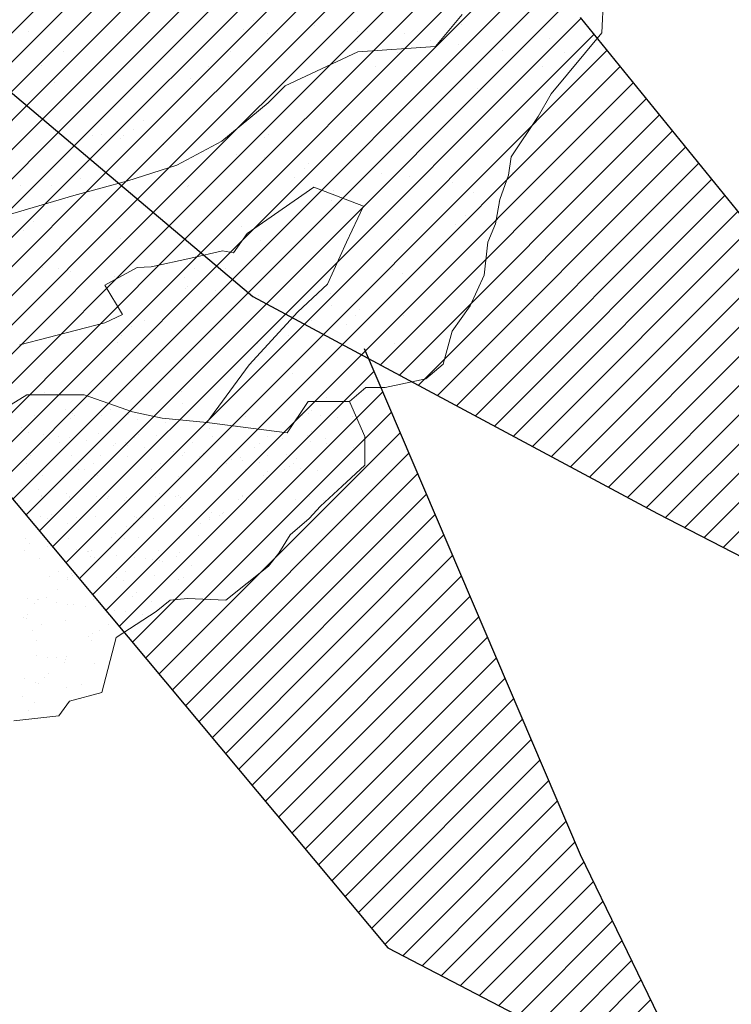
# Model space of a CAD drawing. Units: inches. Extents: x 1986 to 21484, y -1816 to 2016.
# Tile 27 of 85: x 2177.15 to 2182.454, y 1869.056 to 1876.389. Entities that reach past the tile are written whole.
import ezdxf

# ---------------------------------------------------------------- set-up
doc = ezdxf.new("R2010")
doc.units = ezdxf.units.IN
doc.layers.add('L-PLNT', color=84, linetype='Continuous', lineweight=13)
doc.layers.add('vfolhas', color=114, linetype='Continuous', lineweight=5)
doc.layers.add('vfolha', color=72, linetype='Continuous')
doc.layers.add('vfolhas2', color=102, linetype='Continuous')
pattern_1 = [(45, (-2446.5133113, 50.986076), (-0.004419417382, 0.004419417382), [])]

# ---------------------------------------------------------------- blocks, each defined once
blk = doc.blocks.new('arbusto_PB_verde_grande')
at = {"layer": 'vfolhas'}
h = blk.add_hatch(dxfattribs=at)
h.set_pattern_fill('ANSI31', color=256, scale=0.05, style=0)
h.set_pattern_definition(pattern_1)
h.paths.add_polyline_path([(-0.07279, 0.50669), (-0.18085, 0.65063), (-0.2334, 0.67253), (-0.20712, 0.53176), (-0.10785, 0.25007), (0.02625, -0.03934), (0.00028, 0.09048), (0.00816, 0.16241), (-0.04939, 0.29079)])
h.paths.add_polyline_path([(0.09902, 0.41929), (0.09372, 0.26573), (0.07906, 0.18814), (0.15506, 0.36901), (0.26606, 0.5505), (0.28356, 0.63504), (0.2485, 0.68819), (0.25145, 0.63504), (0.20178, 0.54426)])
h.paths.add_polyline_path([(0.12295, 0.24073), (0.047, 0.06233), (0.02625, -0.03934), (0.11122, 0.04358), (0.18428, 0.09364), (0.27478, 0.19376), (0.3215, 0.25323), (0.44129, 0.38467), (0.47634, 0.57866), (0.41789, 0.45347), (0.28939, 0.30954)])
h.paths.add_polyline_path([(0.58145, -0.03779), (0.70707, 0.01536), (0.78591, 0.04667), (0.74796, 0.06549), (0.62818, 0.08423), (0.52595, 0.09048), (0.39745, 0.04358), (0.02625, -0.03934), (0.25728, -0.03154), (0.43834, -0.0347)])
h.paths.add_polyline_path([(0.52022, -0.03647), (0.43834, -0.0347), (0.25728, -0.03154), (0.02625, -0.03934), (0.17964, -0.08515), (0.53768, -0.13167), (0.69541, -0.15357), (0.78591, -0.07852), (0.70413, -0.10042)])
h.paths.add_polyline_path([(0.27189, -0.21929), (0.14922, -0.14107), (0.02625, -0.03934), (0.15794, -0.31007), (0.29522, -0.42585), (0.41789, -0.49157), (0.56396, -0.56669), (0.5114, -0.48532), (0.39456, -0.34139)])
h.paths.add_polyline_path([(-0.05818, -0.47591), (-0.02312, -0.61984), (0.047, -0.80134), (0.08494, -0.59794), (0.07911, -0.4071), (0.03527, -0.25376), (0.02625, -0.03934), (-0.03773, -0.26001)])
h.paths.add_polyline_path([(-0.24218, 0.14054), (-0.11073, 0.06858), (0.02625, -0.03934), (-0.04235, 0.10871), (-0.21007, 0.23757), (-0.36485, 0.33145), (-0.47874, 0.40341), (-0.54303, 0.46288), (-0.49041, 0.33145), (-0.39408, 0.22192)])
h = blk.add_hatch(dxfattribs=at)
h.set_pattern_fill('ANSI31', color=256, scale=0.05, style=0)
h.set_pattern_definition(pattern_1)
h.paths.add_polyline_path([(0.33611, -0.623), (0.43251, -0.67306), (0.39456, -0.59485), (0.3303, -0.44464), (0.29522, -0.42585), (0.15794, -0.31007), (0.14904, -0.29177), (0.18428, -0.44151)])
at = {"layer": 'vfolha'}
for p, q in [((0.15794, -0.31007), (0.29522, -0.42585)), ((0.5114, -0.48532), (0.39456, -0.34139)), ((0.29522, -0.42585), (0.41789, -0.49157)), ((0.41789, -0.49157), (0.56396, -0.56669))]:
    blk.add_line(p, q, dxfattribs=at)
at = {"layer": 'vfolhas2'}
for p, q in [((0.18428, -0.44151), (0.33611, -0.623)), ((0.39456, -0.59485), (0.32904, -0.4417)), ((0.43251, -0.67306), (0.39456, -0.59485)), ((0.33611, -0.623), (0.43251, -0.67306))]:
    blk.add_line(p, q, dxfattribs=at)
blk = doc.blocks.new('PLANT-SHRUB')
for p, q in [((2181.5014, 1876.5696), (2181.4884, 1876.2909)), ((2180.4493, 1876.4278), (2180.2498, 1876.1886)), ((2178.8916, 1876.386), (2178.8916, 1876.386)), ((2179.1367, 1876.3741), (2179.1367, 1876.3741)), ((2180.4407, 1876.3539), (2180.4407, 1876.3539)), ((2177.2186, 1876.3048), (2177.2186, 1876.3048)), ((2177.9529, 1876.2977), (2177.9529, 1876.2977)), ((2178.8179, 1876.3185), (2178.8179, 1876.3185)), ((2178.9991, 1876.2844), (2178.9991, 1876.2844)), ((2179.3447, 1876.3467), (2179.3447, 1876.3467)), ((2179.6696, 1876.304), (2179.6696, 1876.304)), ((2180.0215, 1876.2893), (2180.0215, 1876.2893)), ((2181.4884, 1876.2909), (2181.1123, 1875.8373)), ((2180.2125, 1876.2325), (2180.2125, 1876.2325)), ((2180.4205, 1876.2051), (2180.4205, 1876.2051)), ((2181.101, 1876.2504), (2181.101, 1876.2504)), ((2177.4785, 1876.1519), (2177.4785, 1876.1519)), ((2178.7231, 1876.1496), (2178.7231, 1876.1496)), ((2179.6713, 1876.1487), (2179.1294, 1875.8977)), ((2180.2498, 1876.1886), (2179.6713, 1876.1487)), ((2179.6713, 1876.1487), (2179.6713, 1876.1487)), ((2179.9678, 1876.1474), (2179.9678, 1876.1474)), ((2180.2498, 1876.1886), (2180.2498, 1876.1886)), ((2180.7455, 1876.1623), (2180.7455, 1876.1623)), ((2181.2124, 1876.1451), (2181.2124, 1876.1451)), ((2177.3099, 1876.0445), (2177.3099, 1876.0445)), ((2178.5546, 1876.0423), (2178.5546, 1876.0423)), ((2179.7992, 1876.04), (2179.7992, 1876.04)), ((2180.093, 1876.0352), (2180.093, 1876.0352)), ((2181.0438, 1876.0377), (2181.0438, 1876.0377)), ((2177.4125, 1875.923), (2177.4125, 1875.923)), ((2178.4201, 1875.954), (2178.4201, 1875.954)), ((2178.4349, 1875.9279), (2178.4349, 1875.9279)), ((2180.0194, 1875.9677), (2180.0194, 1875.9677)), ((2179.1294, 1875.8977), (2179.0013, 1875.7697)), ((2179.5143, 1875.889), (2179.5143, 1875.889)), ((2180.5605, 1875.8757), (2180.5605, 1875.8757)), ((2181.1123, 1875.8373), (2181.015, 1875.6688)), ((2181.1123, 1875.8373), (2181.1123, 1875.8373)), ((2179.0013, 1875.7697), (2178.6564, 1875.4842)), ((2178.0724, 1875.6354), (2178.0724, 1875.6354)), ((2181.015, 1875.6688), (2180.8135, 1875.3668)), ((2177.9987, 1875.5679), (2177.9987, 1875.5679)), ((2179.6216, 1875.6032), (2179.6216, 1875.6032)), ((2177.6924, 1875.5295), (2177.6924, 1875.5295)), ((2177.7624, 1875.5376), (2177.7624, 1875.5376)), ((2177.9004, 1875.5021), (2177.9004, 1875.5021)), ((2177.9277, 1875.5276), (2177.9277, 1875.5276)), ((2178.6564, 1875.4842), (2178.3213, 1875.3069)), ((2178.9739, 1875.5143), (2178.9739, 1875.5143)), ((2179.0071, 1875.5353), (2179.0071, 1875.5353)), ((2179.9963, 1875.5192), (2179.9963, 1875.5192)), ((2180.2517, 1875.5331), (2180.2517, 1875.5331)), ((2178.2253, 1875.4593), (2178.2253, 1875.4593)), ((2178.7682, 1875.3878), (2178.7682, 1875.3878)), ((2178.9762, 1875.3605), (2178.9762, 1875.3605)), ((2180.8135, 1875.3668), (2180.794, 1875.2307)), ((2178.3213, 1875.3069), (2177.9567, 1875.1888)), ((2179.2739, 1875.2846), (2179.2739, 1875.2846)), ((2179.3011, 1875.3177), (2179.3011, 1875.3177)), ((2180.823, 1875.2524), (2180.823, 1875.2524)), ((2177.9567, 1875.1888), (2177.5527, 1875.0804)), ((2177.6009, 1875.2034), (2177.6009, 1875.2034)), ((2179.2002, 1875.2171), (2179.2002, 1875.2171)), ((2179.844, 1875.2462), (2179.844, 1875.2462)), ((2180.052, 1875.2188), (2180.052, 1875.2188)), ((2180.377, 1875.176), (2180.377, 1875.176)), ((2180.794, 1875.2307), (2180.7292, 1875.0492)), ((2177.1557, 1875.1511), (2177.1557, 1875.1511)), ((2177.3873, 1875.1529), (2177.3873, 1875.1529)), ((2178.4003, 1875.1488), (2178.4003, 1875.1488)), ((2178.4097, 1875.1578), (2178.4097, 1875.1578)), ((2179.3424, 1875.1428), (2178.8459, 1874.7963)), ((2179.7128, 1875.001), (2179.3424, 1875.1428)), ((2179.4892, 1875.1189), (2179.4892, 1875.1189)), ((2179.645, 1875.1466), (2179.645, 1875.1466)), ((2180.5353, 1875.1056), (2180.5353, 1875.1056)), ((2177.5527, 1875.0804), (2176.8121, 1874.8603)), ((2178.2318, 1875.0414), (2178.2318, 1875.0414)), ((2179.4764, 1875.0392), (2179.4764, 1875.0392)), ((2180.7292, 1875.0492), (2180.6967, 1874.8678)), ((2180.7211, 1875.0369), (2180.7211, 1875.0369)), ((2179.5867, 1874.7333), (2179.7128, 1875.001)), ((2177.2532, 1874.8847), (2177.2532, 1874.8847)), ((2180.4753, 1874.9338), (2180.4753, 1874.9338)), ((2177.1795, 1874.8172), (2177.1795, 1874.8172)), ((2178.8024, 1874.8526), (2178.8024, 1874.8526)), ((2180.4016, 1874.8663), (2180.4016, 1874.8663)), ((2180.6967, 1874.8678), (2180.6384, 1874.7317)), ((2177.9026, 1874.7575), (2177.9026, 1874.7575)), ((2178.8459, 1874.7963), (2178.7436, 1874.6519)), ((2178.8459, 1874.7963), (2178.8459, 1874.7963)), ((2178.9487, 1874.7442), (2178.9487, 1874.7442)), ((2179.9711, 1874.7491), (2179.9711, 1874.7491)), ((2178.6615, 1874.6683), (2178.4262, 1874.6137)), ((2178.7436, 1874.6519), (2178.6615, 1874.6683)), ((2179.4448, 1874.4183), (2179.5867, 1874.7333)), ((2180.6384, 1874.7317), (2180.6124, 1874.4855)), ((2178.4262, 1874.6137), (2178.1307, 1874.548)), ((2177.3239, 1874.5432), (2177.3239, 1874.5432)), ((2177.4397, 1874.5368), (2177.4397, 1874.5368)), ((2177.5319, 1874.5158), (2177.5319, 1874.5158)), ((2178.0267, 1874.5426), (2177.7859, 1874.4113)), ((2178.1307, 1874.548), (2178.0267, 1874.5426)), ((2178.4547, 1874.534), (2178.4547, 1874.534)), ((2178.6843, 1874.5345), (2178.6843, 1874.5345)), ((2179.9289, 1874.5323), (2179.9289, 1874.5323)), ((2177.8568, 1874.473), (2177.8568, 1874.473)), ((2178.381, 1874.4665), (2178.381, 1874.4665)), ((2180.0038, 1874.5018), (2180.0038, 1874.5018)), ((2180.6124, 1874.4855), (2180.5087, 1874.2587)), ((2177.3621, 1874.3828), (2177.3621, 1874.3828)), ((2177.7859, 1874.4113), (2177.9173, 1874.1926)), ((2178.3845, 1874.3877), (2178.3845, 1874.3877)), ((2178.3997, 1874.4015), (2178.3997, 1874.4015)), ((2178.6077, 1874.3742), (2178.6077, 1874.3742)), ((2179.2242, 1874.2136), (2179.4448, 1874.4183)), ((2178.9326, 1874.3314), (2178.9326, 1874.3314)), ((2179.464, 1874.3488), (2179.464, 1874.3488)), ((2179.4755, 1874.2599), (2179.4755, 1874.2599)), ((2179.6835, 1874.2325), (2179.6835, 1874.2325)), ((2180.5087, 1874.2587), (2180.3725, 1874.0707)), ((2177.9173, 1874.1926), (2177.7859, 1874.1325)), ((2178.0775, 1874.148), (2178.0775, 1874.148)), ((2178.8616, 1873.8198), (2179.2242, 1874.2136)), ((2179.6561, 1874.1832), (2179.6561, 1874.1832)), ((2180.0085, 1874.1897), (2180.0085, 1874.1897)), ((2177.7859, 1874.1325), (2177.1512, 1873.9684)), ((2177.9832, 1874.1019), (2177.9832, 1874.1019)), ((2179.3222, 1874.1457), (2179.3222, 1874.1457)), ((2179.5825, 1874.1157), (2179.5825, 1874.1157)), ((2177.909, 1874.0406), (2177.909, 1874.0406)), ((2179.1536, 1874.0384), (2179.1536, 1874.0384)), ((2180.3725, 1874.0707), (2180.3076, 1873.8245)), ((2177.8774, 1873.9874), (2177.8774, 1873.9874)), ((2178.9236, 1873.9741), (2178.9236, 1873.9741)), ((2179.946, 1873.979), (2179.946, 1873.979)), ((2177.6355, 1873.7833), (2177.6355, 1873.7833)), ((2178.5441, 1873.39), (2178.8616, 1873.8198)), ((2180.3076, 1873.8245), (2180.1779, 1873.7143)), ((2180.3076, 1873.8245), (2180.3076, 1873.8245)), ((2177.5618, 1873.7158), (2177.5618, 1873.7158)), ((2179.1847, 1873.7512), (2179.1847, 1873.7512)), ((2180.1779, 1873.7143), (2179.8731, 1873.6495)), ((2179.7304, 1873.6495), (2179.6072, 1873.5458)), ((2179.8731, 1873.6495), (2179.7304, 1873.6495)), ((2177.2044, 1873.5947), (2176.8418, 1873.3742)), ((2177.2044, 1873.5947), (2177.2044, 1873.5947)), ((2177.6299, 1873.5947), (2177.2044, 1873.5947)), ((2177.337, 1873.6127), (2177.337, 1873.6127)), ((2177.9924, 1873.4687), (2177.6299, 1873.5947)), ((2177.6977, 1873.57), (2177.6977, 1873.57)), ((2178.3593, 1873.6176), (2178.3593, 1873.6176)), ((2179.4388, 1873.5787), (2179.4388, 1873.5787)), ((2177.1634, 1873.5295), (2177.1634, 1873.5295)), ((2178.3615, 1873.5337), (2178.3615, 1873.5337)), ((2179.3007, 1873.5458), (2179.1431, 1873.3112)), ((2179.6072, 1873.5458), (2179.3007, 1873.5458)), ((2179.6061, 1873.5315), (2179.6061, 1873.5315)), ((2179.6072, 1873.5458), (2179.7235, 1873.2843)), ((2177.2635, 1873.4415), (2177.2635, 1873.4415)), ((2177.3309, 1873.4844), (2177.3309, 1873.4844)), ((2177.4883, 1873.4867), (2177.4883, 1873.4867)), ((2177.5291, 1873.4156), (2177.5291, 1873.4156)), ((2177.545, 1873.4531), (2177.545, 1873.4531)), ((2177.5586, 1873.4426), (2177.5586, 1873.4426)), ((2177.7614, 1873.4406), (2177.7614, 1873.4406)), ((2177.8288, 1873.4835), (2177.8288, 1873.4835)), ((2177.9634, 1873.4478), (2177.9634, 1873.4478)), ((2178.2131, 1873.4215), (2177.9924, 1873.4687)), ((2178.0312, 1873.4153), (2178.0312, 1873.4153)), ((2178.5441, 1873.39), (2178.2131, 1873.4215)), ((2178.837, 1873.4325), (2178.837, 1873.4325)), ((2179.2226, 1873.4288), (2179.2226, 1873.4288)), ((2179.2549, 1873.4379), (2179.2549, 1873.4379)), ((2179.3055, 1873.4544), (2179.3055, 1873.4544)), ((2179.3223, 1873.4808), (2179.3223, 1873.4808)), ((2179.3887, 1873.4435), (2179.3887, 1873.4435)), ((2179.4671, 1873.4493), (2179.4671, 1873.4493)), ((2179.5187, 1873.4264), (2179.5187, 1873.4264)), ((2179.6316, 1873.4308), (2179.6316, 1873.4308)), ((2177.164, 1873.3513), (2177.164, 1873.3513)), ((2178.2392, 1873.3879), (2178.2392, 1873.3879)), ((2179.1431, 1873.3112), (2178.5441, 1873.39)), ((2178.5641, 1873.3451), (2178.5641, 1873.3451)), ((2178.7633, 1873.365), (2178.7633, 1873.365)), ((2177.2197, 1873.3151), (2177.2197, 1873.3151)), ((2177.3288, 1873.3032), (2177.3288, 1873.3032)), ((2177.37, 1873.2698), (2177.37, 1873.2698)), ((2177.4368, 1873.2865), (2177.4368, 1873.2865)), ((2177.52, 1873.2756), (2177.52, 1873.2756)), ((2177.7377, 1873.3052), (2177.7377, 1873.3052)), ((2178.0097, 1873.2753), (2178.0097, 1873.2753)), ((2178.0392, 1873.3023), (2178.0392, 1873.3023)), ((2178.1695, 1873.2896), (2178.1695, 1873.2896)), ((2178.588, 1873.2843), (2178.588, 1873.2843)), ((2178.6588, 1873.2894), (2178.6588, 1873.2894)), ((2178.997, 1873.2863), (2178.997, 1873.2863)), ((2179.107, 1873.2736), (2179.107, 1873.2736)), ((2179.1431, 1873.3112), (2179.1431, 1873.3112)), ((2179.2985, 1873.2949), (2179.2985, 1873.2949)), ((2179.328, 1873.3219), (2179.328, 1873.3219)), ((2179.4287, 1873.2707), (2179.4287, 1873.2707)), ((2179.7235, 1873.2843), (2179.7235, 1873.0705)), ((2177.4445, 1873.2387), (2177.4445, 1873.2387)), ((2177.65, 1873.2585), (2177.65, 1873.2585)), ((2177.8522, 1873.2174), (2177.8522, 1873.2174)), ((2177.8671, 1873.2299), (2177.8671, 1873.2299)), ((2177.9424, 1873.2378), (2177.9424, 1873.2378)), ((2177.9504, 1873.2189), (2177.9504, 1873.2189)), ((2178.0803, 1873.2018), (2178.0803, 1873.2018)), ((2178.4402, 1873.2369), (2178.4402, 1873.2369)), ((2178.8984, 1873.204), (2178.8984, 1873.204)), ((2178.9381, 1873.236), (2178.9381, 1873.236)), ((2179.315, 1873.2462), (2179.315, 1873.2462)), ((2179.4359, 1873.2351), (2179.4359, 1873.2351)), ((2179.64, 1873.2035), (2179.64, 1873.2035)), ((2177.2309, 1873.1423), (2177.2309, 1873.1423)), ((2177.5349, 1873.1451), (2177.5349, 1873.1451)), ((2177.7548, 1873.1472), (2177.7548, 1873.1472)), ((2177.8506, 1873.1295), (2177.8506, 1873.1295)), ((2177.9534, 1873.1397), (2177.9534, 1873.1397)), ((2178.2975, 1873.1732), (2178.2975, 1873.1732)), ((2178.3623, 1873.1417), (2178.3623, 1873.1417)), ((2178.3807, 1873.1623), (2178.3807, 1873.1623)), ((2178.4903, 1873.1349), (2178.4903, 1873.1349)), ((2178.5107, 1873.1452), (2178.5107, 1873.1452)), ((2178.5198, 1873.1619), (2178.5198, 1873.1619)), ((2178.7941, 1873.1261), (2178.7941, 1873.1261)), ((2178.9994, 1873.1449), (2178.9994, 1873.1449)), ((2179.1394, 1873.1491), (2179.1394, 1873.1491)), ((2177.2014, 1873.1153), (2177.2014, 1873.1153)), ((2177.2018, 1873.0841), (2177.2018, 1873.0841)), ((2177.6997, 1873.0832), (2177.6997, 1873.0832)), ((2178.1975, 1873.0823), (2178.1975, 1873.0823)), ((2178.6954, 1873.0814), (2178.6954, 1873.0814)), ((2178.7278, 1873.1166), (2178.7278, 1873.1166)), ((2178.811, 1873.1056), (2178.811, 1873.1056)), ((2178.941, 1873.0885), (2178.941, 1873.0885)), ((2179.1581, 1873.0599), (2179.1581, 1873.0599)), ((2179.1932, 1873.0805), (2179.1932, 1873.0805)), ((2179.2126, 1873.1208), (2179.2126, 1873.1208)), ((2179.2413, 1873.049), (2179.2413, 1873.049)), ((2179.7235, 1873.0705), (2179.5549, 1872.9149)), ((2177.3187, 1872.9952), (2177.3187, 1872.9952)), ((2177.5862, 1873.0398), (2177.5862, 1873.0398)), ((2177.6323, 1873.0403), (2177.6323, 1873.0403)), ((2177.682, 1872.975), (2177.682, 1872.975)), ((2177.7115, 1873.002), (2177.7115, 1873.002)), ((2177.7277, 1872.9971), (2177.7277, 1872.9971)), ((2178.1301, 1873.0394), (2178.1301, 1873.0394)), ((2178.1595, 1872.9816), (2178.1595, 1872.9816)), ((2178.3312, 1872.9891), (2178.3312, 1872.9891)), ((2178.3655, 1873.0005), (2178.3655, 1873.0005)), ((2178.5779, 1872.9763), (2178.5779, 1872.9763)), ((2178.628, 1873.0384), (2178.628, 1873.0384)), ((2178.8309, 1873.0375), (2178.8309, 1873.0375)), ((2178.9709, 1872.9946), (2178.9709, 1872.9946)), ((2178.9869, 1872.9782), (2178.9869, 1872.9782)), ((2179.0003, 1873.0216), (2179.0003, 1873.0216)), ((2179.1258, 1873.0375), (2179.1258, 1873.0375)), ((2179.3713, 1873.0319), (2179.3713, 1873.0319)), ((2179.5549, 1872.9149), (2179.3928, 1872.7659)), ((2179.4187, 1872.9627), (2179.4187, 1872.9627)), ((2177.2894, 1872.892), (2177.2894, 1872.892)), ((2177.3118, 1872.8426), (2177.3118, 1872.8426)), ((2177.3154, 1872.8384), (2177.3154, 1872.8384)), ((2177.3726, 1872.8811), (2177.3726, 1872.8811)), ((2177.5026, 1872.864), (2177.5026, 1872.864)), ((2177.5229, 1872.8292), (2177.5229, 1872.8292)), ((2177.5248, 1872.837), (2177.5248, 1872.837)), ((2177.7197, 1872.8354), (2177.7197, 1872.8354)), ((2177.8133, 1872.8375), (2177.8133, 1872.8375)), ((2177.9433, 1872.8317), (2177.9433, 1872.8317)), ((2178.1626, 1872.8347), (2178.1626, 1872.8347)), ((2178.1921, 1872.8617), (2178.1921, 1872.8617)), ((2178.3111, 1872.8366), (2178.3111, 1872.8366)), ((2178.3342, 1872.8475), (2178.3342, 1872.8475)), ((2178.3522, 1872.8337), (2178.3522, 1872.8337)), ((2178.809, 1872.8357), (2178.809, 1872.8357)), ((2178.8117, 1872.8488), (2178.8117, 1872.8488)), ((2179.3068, 1872.8348), (2179.3068, 1872.8348)), ((2177.803, 1872.8244), (2177.803, 1872.8244)), ((2177.9329, 1872.8073), (2177.9329, 1872.8073)), ((2178.1501, 1872.7787), (2178.1501, 1872.7787)), ((2178.2333, 1872.7678), (2178.2333, 1872.7678)), ((2178.784, 1872.8181), (2178.784, 1872.8181)), ((2179.2025, 1872.8128), (2179.2025, 1872.8128)), ((2179.3928, 1872.7659), (2179.3085, 1872.6752)), ((2179.4136, 1872.8086), (2179.4136, 1872.8086)), ((2177.3086, 1872.6871), (2177.3086, 1872.6871)), ((2177.3838, 1872.7017), (2177.3838, 1872.7017)), ((2177.5706, 1872.6829), (2177.5706, 1872.6829)), ((2177.7176, 1872.6891), (2177.7176, 1872.6891)), ((2178.0035, 1872.6889), (2178.0035, 1872.6889)), ((2178.0178, 1872.6819), (2178.0178, 1872.6819)), ((2178.0684, 1872.682), (2178.0684, 1872.682)), ((2178.3633, 1872.7506), (2178.3633, 1872.7506)), ((2178.5663, 1872.6811), (2178.5663, 1872.6811)), ((2178.5804, 1872.7221), (2178.5804, 1872.7221)), ((2178.6432, 1872.6944), (2178.6432, 1872.6944)), ((2178.6636, 1872.7111), (2178.6636, 1872.7111)), ((2178.6727, 1872.7214), (2178.6727, 1872.7214)), ((2177.3544, 1872.6747), (2177.3544, 1872.6747)), ((2177.5031, 1872.6399), (2177.5031, 1872.6399)), ((2177.9441, 1872.6144), (2177.9441, 1872.6144)), ((2178.001, 1872.639), (2178.001, 1872.639)), ((2178.1494, 1872.6736), (2178.1494, 1872.6736)), ((2178.4988, 1872.6381), (2178.4988, 1872.6381)), ((2178.5679, 1872.6682), (2178.5679, 1872.6682)), ((2179.3085, 1872.6752), (2179.1658, 1872.552)), ((2177.8349, 1872.5344), (2177.8349, 1872.5344)), ((2177.8644, 1872.5614), (2177.8644, 1872.5614)), ((2178.4841, 1872.5486), (2178.4841, 1872.5486)), ((2179.1658, 1872.552), (2179.0815, 1872.416)), ((2177.1952, 1872.5289), (2177.1952, 1872.5289)), ((2177.2252, 1872.4865), (2177.2252, 1872.4865)), ((2177.3552, 1872.4694), (2177.3552, 1872.4694)), ((2177.5147, 1872.529), (2177.5147, 1872.529)), ((2177.9332, 1872.5237), (2177.9332, 1872.5237)), ((2178.0387, 1872.5329), (2178.0387, 1872.5329)), ((2178.3422, 1872.5256), (2178.3422, 1872.5256)), ((2177.1863, 1872.4381), (2177.1863, 1872.4381)), ((2177.5723, 1872.4409), (2177.5723, 1872.4409)), ((2177.6556, 1872.4299), (2177.6556, 1872.4299)), ((2177.6627, 1872.429), (2177.6627, 1872.429)), ((2177.6758, 1872.3886), (2177.6758, 1872.3886)), ((2177.6841, 1872.4372), (2177.6841, 1872.4372)), ((2177.7855, 1872.4128), (2177.7855, 1872.4128)), ((2177.827, 1872.4473), (2177.827, 1872.4473)), ((2177.8707, 1872.4016), (2177.8707, 1872.4016)), ((2178.182, 1872.4363), (2178.182, 1872.4363)), ((2178.3155, 1872.3941), (2178.3155, 1872.3941)), ((2178.345, 1872.4211), (2178.345, 1872.4211)), ((2179.0815, 1872.416), (2179.0037, 1872.3187)), ((2177.2986, 1872.3791), (2177.2986, 1872.3791)), ((2177.7075, 1872.3811), (2177.7075, 1872.3811)), ((2178.0027, 1872.3842), (2178.0027, 1872.3842)), ((2178.0859, 1872.3732), (2178.0859, 1872.3732)), ((2178.1393, 1872.3655), (2178.1393, 1872.3655)), ((2178.1956, 1872.3588), (2178.1956, 1872.3588)), ((2178.2159, 1872.3561), (2178.2159, 1872.3561)), ((2178.433, 1872.3275), (2178.433, 1872.3275)), ((2179.0037, 1872.3187), (2178.6859, 1872.066)), ((2177.4414, 1872.2826), (2177.4414, 1872.2826)), ((2177.5367, 1872.2612), (2177.5367, 1872.2612)), ((2177.5463, 1872.2499), (2177.5463, 1872.2499)), ((2177.9393, 1872.2816), (2177.9393, 1872.2816)), ((2178.1564, 1872.2483), (2178.1564, 1872.2483)), ((2177.374, 1872.2396), (2177.374, 1872.2396)), ((2177.5047, 1872.221), (2177.5047, 1872.221)), ((2177.5073, 1872.2342), (2177.5073, 1872.2342)), ((2177.8719, 1872.2387), (2177.8719, 1872.2387)), ((2177.9231, 1872.2156), (2177.9231, 1872.2156)), ((2178.3321, 1872.2176), (2178.3321, 1872.2176)), ((2178.3697, 1872.2378), (2178.3697, 1872.2378)), ((2177.432, 1872.1464), (2177.432, 1872.1464)), ((2178.0173, 1872.1209), (2178.0173, 1872.1209)), ((2177.2078, 1872.0749), (2177.2078, 1872.0749)), ((2177.2634, 1872.039), (2177.2634, 1872.039)), ((2177.2866, 1872.0725), (2177.2866, 1872.0725)), ((2177.2885, 1872.0711), (2177.2885, 1872.0711)), ((2177.3482, 1872.0884), (2177.3482, 1872.0884)), ((2177.4249, 1872.0463), (2177.4249, 1872.0463)), ((2177.5082, 1872.0354), (2177.5082, 1872.0354)), ((2177.555, 1872.0368), (2177.555, 1872.0368)), ((2177.6975, 1872.073), (2177.6975, 1872.073)), ((2177.9879, 1872.0939), (2177.9879, 1872.0939)), ((2178.0529, 1872.0359), (2178.0529, 1872.0359)), ((2178.1292, 1872.0575), (2178.1292, 1872.0575)), ((2178.2708, 1872.066), (2178.1671, 1871.9818)), ((2178.4005, 1872.079), (2178.2708, 1872.066)), ((2178.4005, 1872.079), (2178.4005, 1872.079)), ((2178.6859, 1872.066), (2178.4005, 1872.079)), ((2177.2091, 1871.9609), (2177.2091, 1871.9609)), ((2177.6381, 1872.0183), (2177.6381, 1872.0183)), ((2177.8287, 1871.9481), (2177.8287, 1871.9481)), ((2177.8553, 1871.9897), (2177.8553, 1871.9897)), ((2178.1671, 1871.9818), (2177.8688, 1871.7874)), ((2177.9385, 1871.9787), (2177.9385, 1871.9787)), ((2178.0685, 1871.9616), (2178.0685, 1871.9616)), ((2177.1796, 1871.9339), (2177.1796, 1871.9339)), ((2177.1986, 1871.9313), (2177.1986, 1871.9313)), ((2177.3123, 1871.8822), (2177.3123, 1871.8822)), ((2177.4946, 1871.9129), (2177.4946, 1871.9129)), ((2177.8102, 1871.8813), (2177.8102, 1871.8813)), ((2177.9131, 1871.9076), (2177.9131, 1871.9076)), ((2177.2449, 1871.8393), (2177.2449, 1871.8393)), ((2177.6897, 1871.8206), (2177.6897, 1871.8206)), ((2177.7428, 1871.8384), (2177.7428, 1871.8384)), ((2177.2784, 1871.763), (2177.2784, 1871.763)), ((2177.6602, 1871.7936), (2177.6602, 1871.7936)), ((2177.6874, 1871.765), (2177.6874, 1871.765)), ((2177.8688, 1871.7874), (2177.7634, 1871.3785)), ((2177.2775, 1871.6518), (2177.2775, 1871.6518)), ((2177.3608, 1871.6409), (2177.3608, 1871.6409)), ((2177.4259, 1871.6365), (2177.4259, 1871.6365)), ((2177.4845, 1871.6049), (2177.4845, 1871.6049)), ((2177.4907, 1871.6237), (2177.4907, 1871.6237)), ((2177.5011, 1871.6478), (2177.5011, 1871.6478)), ((2177.7079, 1871.5952), (2177.7079, 1871.5952)), ((2177.362, 1871.5204), (2177.362, 1871.5204)), ((2177.1832, 1871.4819), (2177.1832, 1871.4819)), ((2177.2684, 1871.455), (2177.2684, 1871.455)), ((2177.2942, 1871.4427), (2177.2942, 1871.4427)), ((2177.3325, 1871.4934), (2177.3325, 1871.4934)), ((2177.6136, 1871.438), (2177.6136, 1871.438)), ((2177.5022, 1871.4153), (2177.5022, 1871.4153)), ((2177.7634, 1871.3785), (2177.5228, 1871.3129)), ((2177.1734, 1871.3475), (2177.1734, 1871.3475)), ((2177.2614, 1871.3024), (2177.2614, 1871.3024)), ((2177.5228, 1871.3129), (2177.4426, 1871.2036)), ((2177.2134, 1871.2463), (2177.2134, 1871.2463)), ((2177.4426, 1871.2036), (2177.1073, 1871.1672))]:
    blk.add_line(p, q)

msp = doc.modelspace()

# ---------------------------------------------------------------- block references
at = {"layer": 'L-PLNT'}
msp.add_blockref('PLANT-SHRUB', (0, 0), dxfattribs=at)
at = {"layer": 'L-PLNT', "xscale": 24.60366729364114, "yscale": 24.60366729364114, "zscale": 24.60366729364114}
msp.add_blockref('arbusto_PB_verde_grande', (2171.6234, 1884.8051), dxfattribs=at)

doc.saveas('drawing.dxf')
